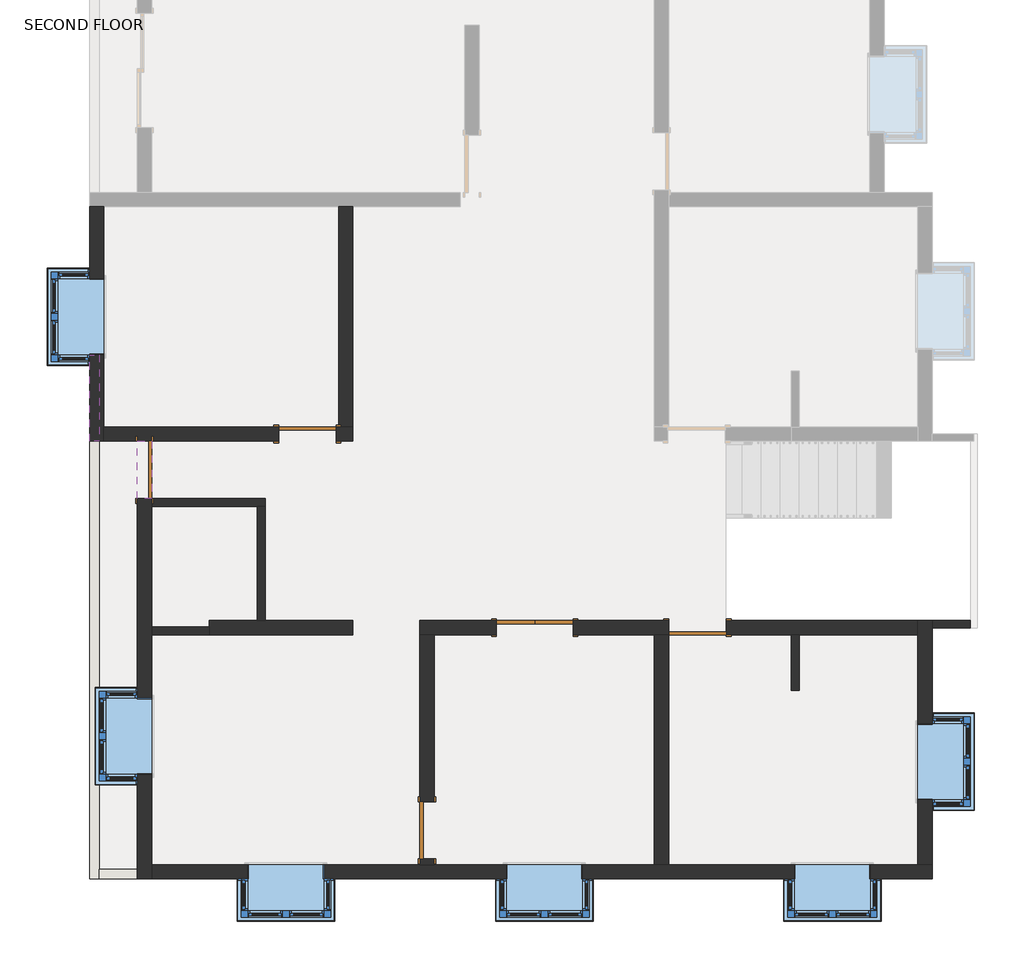
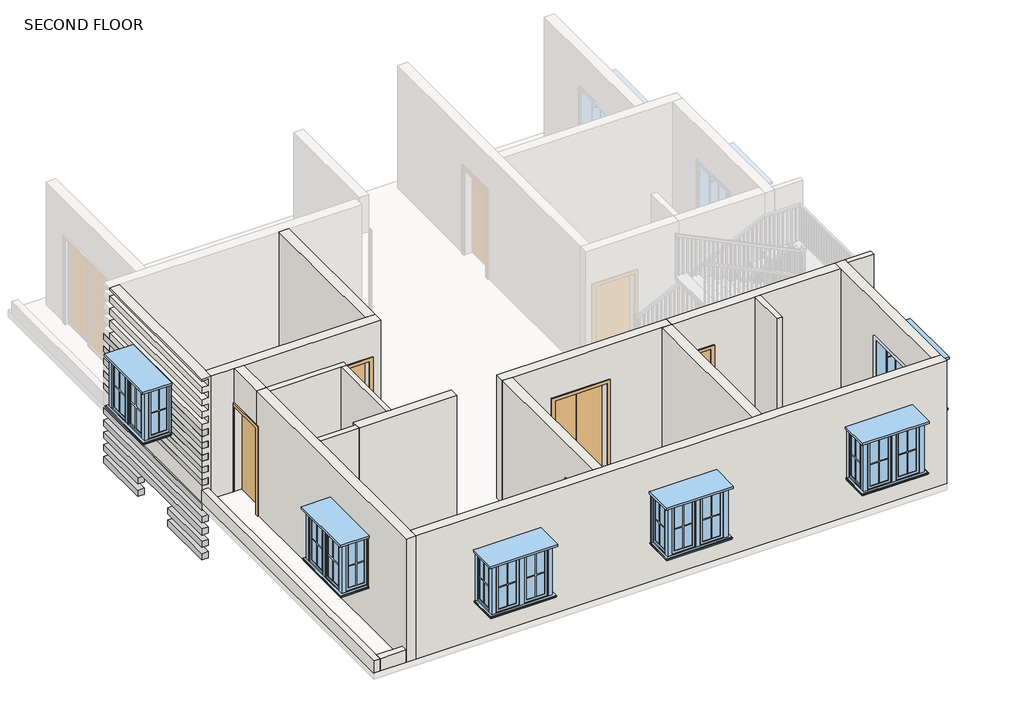
# One storey, part 1 of 6: 19 walls, 10 proxies, 6 windows, 5 doors.
"""IFC4 building model written with IfcOpenShell, lengths in millimetres."""

from ifc_helpers import new_model, si_unit, frame, origin, place, context, project, spatial, polyline, outline, extrude, faceted_brep, transform, mapped, element, save
from components import door_double_flush_panel_4_x7_7c704b5a, door_a90ba1ad, door_0ca8825f, window_bay_casement_box_90_degree_angle_4_x4_x2_07b705a1

model = new_model("IFC4")

# Units and contexts
model_context = context("Model", 3, world=origin())
ifc_project = project(units=[si_unit("LENGTHUNIT", "METRE", prefix="MILLI")], contexts=[model_context])

# Site, building, storey
site = spatial("IfcSite", under=ifc_project)
building = spatial("IfcBuilding", under=site)
storey = spatial("IfcBuildingStorey", under=building, Name="SECOND FLOOR", Elevation=6400.8)

# Proxies
placement = place(None, origin())
element("IfcBuildingElementProxy", 1, Name="Reveal", ObjectType="Reveal", at=placement, inside=storey, context=model_context, shape_type="SweptSolid", body=[
    extrude(outline(polyline([(-7008.3415084, 1592.333346), (-6855.9415084, 1592.333346), (-6855.9415084, 220.733346), (-7008.3415084, 220.733346), (-7008.3415084, 1592.333346)])), frame((0.0, 0.0, 4978.4), z_axis=(0.0, 0.0, 1.0), x_axis=(1.0, 0.0, 0.0)), (0.0, 0.0, 1.0), 152.4),
    extrude(outline(polyline([(-7008.3415084, 4183.133346), (-6855.9415084, 4183.133346), (-6855.9415084, 2811.533346), (-7008.3415084, 2811.533346), (-7008.3415084, 4183.133346)])), frame((0.0, 0.0, 4978.4), z_axis=(0.0, 0.0, 1.0), x_axis=(1.0, 0.0, 0.0)), (0.0, 0.0, 1.0), 152.4),
])
element("IfcBuildingElementProxy", 2, Name="Reveal", ObjectType="Reveal", at=placement, inside=storey, context=model_context, shape_type="SweptSolid", body=[
    extrude(outline(polyline([(-7008.3415084, 1592.333346), (-6855.9415084, 1592.333346), (-6855.9415084, 220.733346), (-7008.3415084, 220.733346), (-7008.3415084, 1592.333346)])), frame((0.0, 0.0, 5283.2), z_axis=(0.0, 0.0, 1.0), x_axis=(1.0, 0.0, 0.0)), (0.0, 0.0, 1.0), 152.4),
    extrude(outline(polyline([(-7008.3415084, 4183.133346), (-6855.9415084, 4183.133346), (-6855.9415084, 2811.533346), (-7008.3415084, 2811.533346), (-7008.3415084, 4183.133346)])), frame((0.0, 0.0, 5283.2), z_axis=(0.0, 0.0, 1.0), x_axis=(1.0, 0.0, 0.0)), (0.0, 0.0, 1.0), 152.4),
])
element("IfcBuildingElementProxy", 3, Name="Reveal", ObjectType="Reveal", at=placement, inside=storey, context=model_context, shape_type="SweptSolid", body=[
    extrude(outline(polyline([(-7008.3415084, 4183.133346), (-6855.9415084, 4183.133346), (-6855.9415084, 220.733346), (-7008.3415084, 220.733346), (-7008.3415084, 4183.133346)])), frame((0.0, 0.0, 5588.0), z_axis=(0.0, 0.0, 1.0), x_axis=(1.0, 0.0, 0.0)), (0.0, 0.0, 1.0), 152.4),
])
element("IfcBuildingElementProxy", 4, Name="Reveal", ObjectType="Reveal", at=placement, inside=storey, context=model_context, shape_type="SweptSolid", body=[
    extrude(outline(polyline([(-7008.3415084, 4183.133346), (-6855.9415084, 4183.133346), (-6855.9415084, 220.733346), (-7008.3415084, 220.733346), (-7008.3415084, 4183.133346)])), frame((0.0, 0.0, 5892.8), z_axis=(0.0, 0.0, 1.0), x_axis=(1.0, 0.0, 0.0)), (0.0, 0.0, 1.0), 152.4),
])
element("IfcBuildingElementProxy", 5, Name="Reveal", ObjectType="Reveal", at=placement, inside=storey, context=model_context, shape_type="SweptSolid", body=[
    extrude(outline(polyline([(-7008.3415084, 4183.133346), (-6855.9415084, 4183.133346), (-6855.9415084, 220.733346), (-7008.3415084, 220.733346), (-7008.3415084, 4183.133346)])), frame((0.0, 0.0, 6197.6), z_axis=(0.0, 0.0, 1.0), x_axis=(1.0, 0.0, 0.0)), (0.0, 0.0, 1.0), 152.4),
])
element("IfcBuildingElementProxy", 6, Name="Reveal", ObjectType="Reveal", at=placement, inside=storey, context=model_context, shape_type="SweptSolid", body=[
    extrude(outline(polyline([(-7008.3415084, 4183.133346), (-6855.9415084, 4183.133346), (-6855.9415084, 220.733346), (-7008.3415084, 220.733346), (-7008.3415084, 4183.133346)])), frame((0.0, 0.0, 6807.2), z_axis=(0.0, 0.0, 1.0), x_axis=(1.0, 0.0, 0.0)), (0.0, 0.0, 1.0), 152.4),
])
element("IfcBuildingElementProxy", 7, Name="Reveal", ObjectType="Reveal", at=placement, inside=storey, context=model_context, shape_type="SweptSolid", body=[
    extrude(outline(polyline([(-7008.3415084, 4183.133346), (-6855.9415084, 4183.133346), (-6855.9415084, 220.733346), (-7008.3415084, 220.733346), (-7008.3415084, 4183.133346)])), frame((0.0, 0.0, 7112.0), z_axis=(0.0, 0.0, 1.0), x_axis=(1.0, 0.0, 0.0)), (0.0, 0.0, 1.0), 152.4),
])
element("IfcBuildingElementProxy", 8, Name="Reveal", ObjectType="Reveal", at=placement, inside=storey, context=model_context, shape_type="SweptSolid", body=[
    extrude(outline(polyline([(-7008.3415084, 1592.333346), (-6855.9415084, 1592.333346), (-6855.9415084, 220.733346), (-7008.3415084, 220.733346), (-7008.3415084, 1592.333346)])), frame((0.0, 0.0, 7416.8), z_axis=(0.0, 0.0, 1.0), x_axis=(1.0, 0.0, 0.0)), (0.0, 0.0, 1.0), 152.4),
    extrude(outline(polyline([(-7008.3415084, 4183.133346), (-6855.9415084, 4183.133346), (-6855.9415084, 2811.533346), (-7008.3415084, 2811.533346), (-7008.3415084, 4183.133346)])), frame((0.0, 0.0, 7416.8), z_axis=(0.0, 0.0, 1.0), x_axis=(1.0, 0.0, 0.0)), (0.0, 0.0, 1.0), 152.4),
])
element("IfcBuildingElementProxy", 9, Name="Reveal", ObjectType="Reveal", at=placement, inside=storey, context=model_context, shape_type="SweptSolid", body=[
    extrude(outline(polyline([(-7008.3415084, 1592.333346), (-6855.9415084, 1592.333346), (-6855.9415084, 220.733346), (-7008.3415084, 220.733346), (-7008.3415084, 1592.333346)])), frame((0.0, 0.0, 7721.6), z_axis=(0.0, 0.0, 1.0), x_axis=(1.0, 0.0, 0.0)), (0.0, 0.0, 1.0), 152.4),
    extrude(outline(polyline([(-7008.3415084, 4183.133346), (-6855.9415084, 4183.133346), (-6855.9415084, 2811.533346), (-7008.3415084, 2811.533346), (-7008.3415084, 4183.133346)])), frame((0.0, 0.0, 7721.6), z_axis=(0.0, 0.0, 1.0), x_axis=(1.0, 0.0, 0.0)), (0.0, 0.0, 1.0), 152.4),
])
element("IfcBuildingElementProxy", 10, Name="Reveal", ObjectType="Reveal", at=placement, inside=storey, context=model_context, shape_type="SweptSolid", body=[
    extrude(outline(polyline([(-7008.3415084, 1592.333346), (-6855.9415084, 1592.333346), (-6855.9415084, 220.733346), (-7008.3415084, 220.733346), (-7008.3415084, 1592.333346)])), frame((0.0, 0.0, 8026.4), z_axis=(0.0, 0.0, 1.0), x_axis=(1.0, 0.0, 0.0)), (0.0, 0.0, 1.0), 152.4),
    extrude(outline(polyline([(-7008.3415084, 4183.133346), (-6855.9415084, 4183.133346), (-6855.9415084, 2811.533346), (-7008.3415084, 2811.533346), (-7008.3415084, 4183.133346)])), frame((0.0, 0.0, 8026.4), z_axis=(0.0, 0.0, 1.0), x_axis=(1.0, 0.0, 0.0)), (0.0, 0.0, 1.0), 152.4),
])

# Doors
door_double_flush_panel_4_x7_shape = door_double_flush_panel_4_x7_7c704b5a(model_context)
element("IfcDoor", 11, ObjectType="Door-Double-Flush_Panel : 4'x7'", at=placement, inside=storey, context=model_context, shape_type="MappedRepresentation", body=[
    mapped(door_double_flush_panel_4_x7_shape, transform((78.2584916, -2751.066654, 6400.8), x_axis=(1.0, 0.0, 0.0), y_axis=(0.0, 1.0, 0.0), z_axis=(0.0, 0.0, 1.0))),
])
door_shape = door_a90ba1ad(model_context)
element("IfcDoor", 12, ObjectType="Single-Flush : 36\" x 84\"", at=placement, inside=storey, context=model_context, shape_type="MappedRepresentation", body=[
    mapped(door_shape, transform((-1636.2415084, -5976.866654, 6400.8), x_axis=(0.0, -1.0, 0.0), y_axis=(1.0, 0.0, 0.0), z_axis=(0.0, 0.0, 1.0))),
])
door_2_shape = door_0ca8825f(model_context)
element("IfcDoor", 13, ObjectType="Single-Flush : 36\" x 84\"", at=placement, inside=storey, context=model_context, shape_type="MappedRepresentation", body=[
    mapped(door_2_shape, transform((-3541.2415084, 335.033346, 6400.8), x_axis=(1.0, 0.0, 0.0), y_axis=(0.0, 1.0, 0.0), z_axis=(0.0, 0.0, 1.0))),
])
element("IfcDoor", 14, ObjectType="Single-Flush : 36\" x 84\"", at=placement, inside=storey, context=model_context, shape_type="MappedRepresentation", body=[
    mapped(door_2_shape, transform((2669.0584916, -2751.066654, 6400.8), x_axis=(-1.0, 0.0, 0.0), y_axis=(0.0, -1.0, 0.0), z_axis=(0.0, 0.0, 1.0))),
])
element("IfcDoor", 15, ObjectType="Single-Flush : 36\" x 84\"", at=placement, inside=storey, context=model_context, shape_type="MappedRepresentation", body=[
    mapped(door_2_shape, transform((-6132.0415084, -236.466654, 6400.8), x_axis=(0.0, -1.0, 0.0), y_axis=(1.0, 0.0, 0.0), z_axis=(0.0, 0.0, 1.0))),
])

# Walls
element("IfcWall", 16, ObjectType="4.6\"", at=placement, inside=storey, context=model_context, shape_type="SweptSolid", body=[
    extrude(outline(polyline([(7009.1350459, -2753.606654), (6402.8584916, -2753.606654), (6402.8584916, -2636.766654), (7009.1350459, -2636.766654), (7009.1350459, -2753.606654)])), frame((0.0, 0.0, 6400.8), z_axis=(0.0, 0.0, 1.0), x_axis=(1.0, 0.0, 0.0)), (0.0, 0.0, 1.0), 3048.0),
])
element("IfcWall", 17, ObjectType="5\"", at=placement, inside=storey, context=model_context, shape_type="SweptSolid", body=[
    extrude(outline(polyline([(4159.1868368, -3751.826654), (4159.1868368, -2865.366654), (4286.1868368, -2865.366654), (4286.1868368, -3751.826654), (4159.1868368, -3751.826654)])), frame((0.0, 0.0, 6400.8), z_axis=(0.0, 0.0, 1.0), x_axis=(1.0, 0.0, 0.0)), (0.0, 0.0, 1.0), 3048.0),
])
element("IfcWall", 18, ObjectType="5\"", at=placement, inside=storey, context=model_context, shape_type="Brep", body=[
    faceted_brep([(-6017.7415084, -820.666654, 6400.8), (-4341.3415084, -820.666654, 6400.8), (-4214.3415084, -820.666654, 6400.8), (-4214.3415084, -820.666654, 9448.8), (-4341.3415084, -820.666654, 9448.8), (-6017.7415084, -820.666654, 9448.8), (-6017.7415084, -693.666654, 6400.8), (-6017.7415084, -693.666654, 9448.8), (-4214.3415084, -693.666654, 9448.8), (-4214.3415084, -693.666654, 6400.8)], [[[0, 1, 2, 3, 4, 5]], [[6, 7, 8, 9]], [[2, 1, 0, 6, 9]], [[5, 4, 3, 8, 7]], [[0, 5, 7, 6]], [[3, 2, 9, 8]]]),
])
element("IfcWall", 19, ObjectType="5\"", at=placement, inside=storey, context=model_context, shape_type="SweptSolid", body=[
    extrude(outline(polyline([(-4341.3415084, -2636.766654), (-4341.3415084, -820.666654), (-4214.3415084, -820.666654), (-4214.3415084, -2636.766654), (-4341.3415084, -2636.766654)])), frame((0.0, 0.0, 6400.8), z_axis=(0.0, 0.0, 1.0), x_axis=(1.0, 0.0, 0.0)), (0.0, 0.0, 1.0), 3048.0),
])
element("IfcWall", 20, ObjectType="5\"", at=placement, inside=storey, context=model_context, shape_type="SweptSolid", body=[
    extrude(outline(polyline([(-6017.7415084, -2738.366654), (-5103.3415084, -2738.366654), (-5103.3415084, -2865.366654), (-6017.7415084, -2865.366654), (-6017.7415084, -2738.366654)])), frame((0.0, 0.0, 6400.8), z_axis=(0.0, 0.0, 1.0), x_axis=(1.0, 0.0, 0.0)), (0.0, 0.0, 1.0), 3048.0),
])
element("IfcWall", 21, ObjectType="6\"", at=placement, inside=storey, context=model_context, shape_type="Brep", body=[
    faceted_brep([(-7008.3415084, 220.733346, 6400.8), (-7008.3415084, -6751.566654, 6400.8), (-7008.3415084, -6751.566654, 6705.6), (-7008.3415084, 220.733346, 6705.6), (-6855.9415084, 220.733346, 6400.8), (-6855.9415084, 220.733346, 6705.6), (-6855.9415084, -6599.166654, 6705.6), (-6855.9415084, -6751.566654, 6705.6), (-6855.9415084, -6751.566654, 6400.8), (-6855.9415084, -6599.166654, 6400.8)], [[[0, 1, 2, 3]], [[4, 5, 6, 7, 8, 9]], [[1, 0, 4, 9, 8]], [[3, 2, 7, 6, 5]], [[2, 1, 8, 7]], [[0, 3, 5, 4]]]),
])
element("IfcWall", 22, ObjectType="6\"", at=placement, inside=storey, context=model_context, shape_type="SweptSolid", body=[
    extrude(outline(polyline([(-6246.3415084, -6751.566654), (-6855.9415084, -6751.566654), (-6855.9415084, -6599.166654), (-6246.3415084, -6599.166654), (-6246.3415084, -6751.566654)])), frame((0.0, 0.0, 6400.8), z_axis=(0.0, 0.0, 1.0), x_axis=(1.0, 0.0, 0.0)), (0.0, 0.0, 1.0), 304.8),
])
element("IfcWall", 23, ObjectType="9\"", at=placement, inside=storey, context=model_context, shape_type="Brep", body=[
    faceted_brep([(-7008.3415084, 3954.533346, 6400.8), (-7008.3415084, 220.733346, 6400.8), (-7008.3415084, 220.733346, 6705.6), (-7008.3415084, 220.733346, 6807.2), (-7008.3415084, 3954.533346, 6807.2), (-7008.3415084, 220.733346, 9448.8), (-7008.3415084, 3954.533346, 9448.8), (-7008.3415084, 3954.533346, 9398.0), (-7008.3415084, 220.733346, 9398.0), (-7008.3415084, 1592.333346, 7315.2), (-7008.3415084, 2811.533346, 7315.2), (-7008.3415084, 2811.533346, 7416.8), (-7008.3415084, 3954.533346, 7416.8), (-7008.3415084, 3954.533346, 7264.4), (-7008.3415084, 220.733346, 7264.4), (-7008.3415084, 220.733346, 7416.8), (-7008.3415084, 1592.333346, 7416.8), (-7008.3415084, 2811.533346, 8585.2), (-7008.3415084, 1592.333346, 8585.2), (-7008.3415084, 1592.333346, 8483.6), (-7008.3415084, 220.733346, 8483.6), (-7008.3415084, 220.733346, 8636.0), (-7008.3415084, 3954.533346, 8636.0), (-7008.3415084, 3954.533346, 8483.6), (-7008.3415084, 2811.533346, 8483.6), (-7008.3415084, 220.733346, 9245.6), (-7008.3415084, 3954.533346, 9245.6), (-7008.3415084, 3954.533346, 9093.2), (-7008.3415084, 220.733346, 9093.2), (-7008.3415084, 220.733346, 8940.8), (-7008.3415084, 3954.533346, 8940.8), (-7008.3415084, 3954.533346, 8788.4), (-7008.3415084, 220.733346, 8788.4), (-7008.3415084, 220.733346, 8331.2), (-7008.3415084, 1592.333346, 8331.2), (-7008.3415084, 1592.333346, 8178.8), (-7008.3415084, 220.733346, 8178.8), (-7008.3415084, 2811.533346, 8331.2), (-7008.3415084, 3954.533346, 8331.2), (-7008.3415084, 3954.533346, 8178.8), (-7008.3415084, 2811.533346, 8178.8), (-7008.3415084, 220.733346, 8026.4), (-7008.3415084, 1592.333346, 8026.4), (-7008.3415084, 1592.333346, 7874.0), (-7008.3415084, 220.733346, 7874.0), (-7008.3415084, 2811.533346, 8026.4), (-7008.3415084, 3954.533346, 8026.4), (-7008.3415084, 3954.533346, 7874.0), (-7008.3415084, 2811.533346, 7874.0), (-7008.3415084, 220.733346, 7721.6), (-7008.3415084, 1592.333346, 7721.6), (-7008.3415084, 1592.333346, 7569.2), (-7008.3415084, 220.733346, 7569.2), (-7008.3415084, 2811.533346, 7721.6), (-7008.3415084, 3954.533346, 7721.6), (-7008.3415084, 3954.533346, 7569.2), (-7008.3415084, 2811.533346, 7569.2), (-7008.3415084, 220.733346, 7112.0), (-7008.3415084, 3954.533346, 7112.0), (-7008.3415084, 3954.533346, 6959.6), (-7008.3415084, 220.733346, 6959.6), (-6779.7415084, 220.733346, 6400.8), (-6779.7415084, 449.333346, 6400.8), (-6779.7415084, 3954.533346, 6400.8), (-6779.7415084, 3954.533346, 9448.8), (-6779.7415084, 449.333346, 9448.8), (-6779.7415084, 220.733346, 9448.8), (-6779.7415084, 2811.533346, 8585.2), (-6779.7415084, 2811.533346, 7315.2), (-6779.7415084, 1592.333346, 7315.2), (-6779.7415084, 1592.333346, 8585.2), (-6855.9415084, 220.733346, 6400.8), (-6855.9415084, 2811.533346, 8483.6), (-6855.9415084, 2811.533346, 8331.2), (-6855.9415084, 2811.533346, 8178.8), (-6855.9415084, 2811.533346, 8026.4), (-6855.9415084, 2811.533346, 7874.0), (-6855.9415084, 2811.533346, 7721.6), (-6855.9415084, 2811.533346, 7569.2), (-6855.9415084, 2811.533346, 7416.8), (-6855.9415084, 1592.333346, 7416.8), (-6855.9415084, 1592.333346, 7569.2), (-6855.9415084, 1592.333346, 7721.6), (-6855.9415084, 1592.333346, 7874.0), (-6855.9415084, 1592.333346, 8026.4), (-6855.9415084, 1592.333346, 8178.8), (-6855.9415084, 1592.333346, 8331.2), (-6855.9415084, 1592.333346, 8483.6), (-6855.9415084, 220.733346, 9398.0), (-6855.9415084, 220.733346, 9245.6), (-6855.9415084, 220.733346, 9093.2), (-6855.9415084, 220.733346, 8940.8), (-6855.9415084, 220.733346, 8788.4), (-6855.9415084, 220.733346, 8636.0), (-6855.9415084, 220.733346, 8483.6), (-6855.9415084, 220.733346, 8331.2), (-6855.9415084, 220.733346, 8178.8), (-6855.9415084, 220.733346, 8026.4), (-6855.9415084, 220.733346, 7874.0), (-6855.9415084, 220.733346, 7721.6), (-6855.9415084, 220.733346, 7569.2), (-6855.9415084, 220.733346, 7416.8), (-6855.9415084, 220.733346, 7264.4), (-6855.9415084, 220.733346, 7112.0), (-6855.9415084, 220.733346, 6959.6), (-6855.9415084, 220.733346, 6807.2), (-6855.9415084, 3954.533346, 6807.2), (-6855.9415084, 3954.533346, 6959.6), (-6855.9415084, 3954.533346, 7112.0), (-6855.9415084, 3954.533346, 7264.4), (-6855.9415084, 3954.533346, 7416.8), (-6855.9415084, 3954.533346, 7569.2), (-6855.9415084, 3954.533346, 7721.6), (-6855.9415084, 3954.533346, 7874.0), (-6855.9415084, 3954.533346, 8026.4), (-6855.9415084, 3954.533346, 8178.8), (-6855.9415084, 3954.533346, 8331.2), (-6855.9415084, 3954.533346, 8483.6), (-6855.9415084, 3954.533346, 8636.0), (-6855.9415084, 3954.533346, 8788.4), (-6855.9415084, 3954.533346, 8940.8), (-6855.9415084, 3954.533346, 9093.2), (-6855.9415084, 3954.533346, 9245.6), (-6855.9415084, 3954.533346, 9398.0)], [[[0, 1, 2, 3, 4]], [[5, 6, 7, 8]], [[9, 10, 11, 12, 13, 14, 15, 16]], [[17, 18, 19, 20, 21, 22, 23, 24]], [[25, 26, 27, 28]], [[29, 30, 31, 32]], [[33, 34, 35, 36]], [[37, 38, 39, 40]], [[41, 42, 43, 44]], [[45, 46, 47, 48]], [[49, 50, 51, 52]], [[53, 54, 55, 56]], [[57, 58, 59, 60]], [[61, 62, 63, 64, 65, 66], [67, 68, 69, 70]], [[1, 0, 63, 62, 61, 71]], [[6, 5, 66, 65, 64]], [[68, 67, 17, 24, 72, 73, 37, 40, 74, 75, 45, 48, 76, 77, 53, 56, 78, 79, 11, 10]], [[69, 68, 10, 9]], [[70, 69, 9, 16, 80, 81, 51, 50, 82, 83, 43, 42, 84, 85, 35, 34, 86, 87, 19, 18]], [[67, 70, 18, 17]], [[1, 71, 61, 66, 5, 8, 88, 89, 25, 28, 90, 91, 29, 32, 92, 93, 21, 20, 94, 95, 33, 36, 96, 97, 41, 44, 98, 99, 49, 52, 100, 101, 15, 14, 102, 103, 57, 60, 104, 105, 3, 2]], [[6, 64, 63, 0, 4, 106, 107, 59, 58, 108, 109, 13, 12, 110, 111, 55, 54, 112, 113, 47, 46, 114, 115, 39, 38, 116, 117, 23, 22, 118, 119, 31, 30, 120, 121, 27, 26, 122, 123, 7]], [[123, 88, 8, 7]], [[88, 123, 122, 89]], [[89, 122, 26, 25]], [[121, 90, 28, 27]], [[90, 121, 120, 91]], [[91, 120, 30, 29]], [[119, 92, 32, 31]], [[92, 119, 118, 93]], [[93, 118, 22, 21]], [[87, 94, 20, 19]], [[94, 87, 86, 95]], [[95, 86, 34, 33]], [[117, 72, 24, 23]], [[72, 117, 116, 73]], [[73, 116, 38, 37]], [[85, 96, 36, 35]], [[96, 85, 84, 97]], [[97, 84, 42, 41]], [[115, 74, 40, 39]], [[74, 115, 114, 75]], [[75, 114, 46, 45]], [[83, 98, 44, 43]], [[98, 83, 82, 99]], [[99, 82, 50, 49]], [[113, 76, 48, 47]], [[76, 113, 112, 77]], [[77, 112, 54, 53]], [[81, 100, 52, 51]], [[100, 81, 80, 101]], [[101, 80, 16, 15]], [[111, 78, 56, 55]], [[78, 111, 110, 79]], [[79, 110, 12, 11]], [[109, 102, 14, 13]], [[102, 109, 108, 103]], [[103, 108, 58, 57]], [[107, 104, 60, 59]], [[104, 107, 106, 105]], [[105, 106, 4, 3]]]),
])
element("IfcWall", 24, ObjectType="9\"", at=placement, inside=storey, context=model_context, shape_type="Brep", body=[
    faceted_brep([(-3084.0415084, 220.733346, 8534.4), (-3084.0415084, 220.733346, 6400.8), (-2817.3415084, 220.733346, 6400.8), (-2817.3415084, 220.733346, 9448.8), (-6017.7415084, 220.733346, 9448.8), (-6246.3415084, 220.733346, 9448.8), (-6779.7415084, 220.733346, 9448.8), (-6779.7415084, 220.733346, 6400.8), (-3998.4415084, 220.733346, 6400.8), (-3998.4415084, 220.733346, 8534.4), (-2817.3415084, 449.333346, 6400.8), (-3045.9415084, 449.333346, 6400.8), (-3084.0415084, 449.333346, 6400.8), (-3084.0415084, 449.333346, 8534.4), (-3998.4415084, 449.333346, 8534.4), (-3998.4415084, 449.333346, 6400.8), (-6779.7415084, 449.333346, 6400.8), (-6779.7415084, 449.333346, 9448.8), (-3045.9415084, 449.333346, 9448.8), (-2817.3415084, 449.333346, 9448.8)], [[[0, 1, 2, 3, 4, 5, 6, 7, 8, 9]], [[10, 11, 12, 13, 14, 15, 16, 17, 18, 19]], [[8, 7, 16, 15]], [[2, 1, 12, 11, 10]], [[6, 5, 4, 3, 19, 18, 17]], [[3, 2, 10, 19]], [[13, 12, 1, 0]], [[14, 13, 0, 9]], [[15, 14, 9, 8]], [[6, 17, 16, 7]]]),
])
element("IfcWall", 25, ObjectType="9\"", at=placement, inside=storey, context=model_context, shape_type="SweptSolid", body=[
    extrude(outline(polyline([(-2817.3415084, 3954.533346), (-2817.3415084, 449.333346), (-3045.9415084, 449.333346), (-3045.9415084, 3954.533346), (-2817.3415084, 3954.533346)])), frame((0.0, 0.0, 6400.8), z_axis=(0.0, 0.0, 1.0), x_axis=(1.0, 0.0, 0.0)), (0.0, 0.0, 1.0), 3048.0),
])
element("IfcWall", 26, ObjectType="9\"", at=placement, inside=storey, context=model_context, shape_type="Brep", body=[
    faceted_brep([(-6246.3415084, -693.666654, 6400.8), (-6246.3415084, -6599.166654, 6400.8), (-6246.3415084, -6751.566654, 6400.8), (-6246.3415084, -6751.566654, 6705.6), (-6246.3415084, -6751.566654, 9448.8), (-6246.3415084, -693.666654, 9448.8), (-6246.3415084, -693.666654, 8534.4), (-6246.3415084, -3868.666654, 8585.2), (-6246.3415084, -5087.866654, 8585.2), (-6246.3415084, -5087.866654, 7315.2), (-6246.3415084, -3868.666654, 7315.2), (-6017.7415084, -693.666654, 6400.8), (-6017.7415084, -693.666654, 8534.4), (-6017.7415084, -693.666654, 9448.8), (-6017.7415084, -820.666654, 9448.8), (-6017.7415084, -2738.366654, 9448.8), (-6017.7415084, -2865.366654, 9448.8), (-6017.7415084, -6522.966654, 9448.8), (-6017.7415084, -6751.566654, 9448.8), (-6017.7415084, -6751.566654, 6400.8), (-6017.7415084, -6522.966654, 6400.8), (-6017.7415084, -2865.366654, 6400.8), (-6017.7415084, -2738.366654, 6400.8), (-6017.7415084, -820.666654, 6400.8), (-6017.7415084, -3868.666654, 8585.2), (-6017.7415084, -3868.666654, 7315.2), (-6017.7415084, -5087.866654, 7315.2), (-6017.7415084, -5087.866654, 8585.2)], [[[0, 1, 2, 3, 4, 5, 6], [7, 8, 9, 10]], [[11, 12, 13, 14, 15, 16, 17, 18, 19, 20, 21, 22, 23], [24, 25, 26, 27]], [[2, 1, 0, 11, 23, 22, 21, 20, 19]], [[5, 4, 18, 17, 16, 15, 14, 13]], [[0, 6, 5, 13, 12, 11]], [[25, 24, 7, 10]], [[26, 25, 10, 9]], [[27, 26, 9, 8]], [[24, 27, 8, 7]], [[2, 19, 18, 4, 3]]]),
])
element("IfcWall", 27, ObjectType="9\"", at=placement, inside=storey, context=model_context, shape_type="Brep", body=[
    faceted_brep([(-2817.3415084, -2636.766654, 6400.8), (-4214.3415084, -2636.766654, 6400.8), (-4341.3415084, -2636.766654, 6400.8), (-5103.3415084, -2636.766654, 6400.8), (-5103.3415084, -2636.766654, 9448.8), (-4341.3415084, -2636.766654, 9448.8), (-4214.3415084, -2636.766654, 9448.8), (-2817.3415084, -2636.766654, 9448.8), (-2817.3415084, -2865.366654, 6400.8), (-2817.3415084, -2865.366654, 9448.8), (-5103.3415084, -2865.366654, 9448.8), (-5103.3415084, -2865.366654, 6400.8), (-5103.3415084, -2738.366654, 6400.8), (-5103.3415084, -2738.366654, 9448.8)], [[[0, 1, 2, 3, 4, 5, 6, 7]], [[8, 9, 10, 11]], [[3, 2, 1, 0, 8, 11, 12]], [[4, 3, 12, 11, 10, 13]], [[7, 6, 5, 4, 13, 10, 9]], [[0, 7, 9, 8]]]),
])
element("IfcWall", 28, ObjectType="9\"", at=placement, inside=storey, context=model_context, shape_type="Brep", body=[
    faceted_brep([(2211.8584916, -2865.366654, 9448.8), (1983.2584916, -2865.366654, 9448.8), (-1521.9415084, -2865.366654, 9448.8), (-1750.5415084, -2865.366654, 9448.8), (-1750.5415084, -2865.366654, 6400.8), (-1521.9415084, -2865.366654, 6400.8), (-531.3415084, -2865.366654, 6400.8), (-531.3415084, -2865.366654, 8534.4), (687.8584916, -2865.366654, 8534.4), (687.8584916, -2865.366654, 6400.8), (1983.2584916, -2865.366654, 6400.8), (2211.8584916, -2865.366654, 6400.8), (2211.8584916, -2865.366654, 8534.4), (-1750.5415084, -2636.766654, 9448.8), (2211.8584916, -2636.766654, 9448.8), (2211.8584916, -2636.766654, 8534.4), (2211.8584916, -2636.766654, 6400.8), (687.8584916, -2636.766654, 6400.8), (687.8584916, -2636.766654, 8534.4), (-531.3415084, -2636.766654, 8534.4), (-531.3415084, -2636.766654, 6400.8), (-1750.5415084, -2636.766654, 6400.8)], [[[0, 1, 2, 3, 4, 5, 6, 7, 8, 9, 10, 11, 12]], [[13, 14, 15, 16, 17, 18, 19, 20, 21]], [[16, 11, 10, 9, 17]], [[4, 21, 20, 6, 5]], [[3, 2, 1, 0, 14, 13]], [[0, 12, 11, 16, 15, 14]], [[4, 3, 13, 21]], [[8, 18, 17, 9]], [[18, 8, 7, 19]], [[19, 7, 6, 20]]]),
])
element("IfcWall", 29, ObjectType="9\"", at=placement, inside=storey, context=model_context, shape_type="SweptSolid", body=[
    extrude(outline(polyline([(1983.2584916, -6522.966654), (1983.2584916, -2865.366654), (2211.8584916, -2865.366654), (2211.8584916, -6522.966654), (1983.2584916, -6522.966654)])), frame((0.0, 0.0, 6400.8), z_axis=(0.0, 0.0, 1.0), x_axis=(1.0, 0.0, 0.0)), (0.0, 0.0, 1.0), 3048.0),
])
element("IfcWall", 30, ObjectType="9\"", at=placement, inside=storey, context=model_context, shape_type="Brep", body=[
    faceted_brep([(-6017.7415084, -6751.566654, 9448.8), (-6017.7415084, -6751.566654, 6400.8), (6402.8584916, -6751.566654, 6400.8), (6402.8584916, -6751.566654, 9448.8), (-378.9415084, -6751.566654, 8585.2), (840.2584916, -6751.566654, 8585.2), (840.2584916, -6751.566654, 7315.2), (-378.9415084, -6751.566654, 7315.2), (4205.7584916, -6751.566654, 8585.2), (5424.9584916, -6751.566654, 8585.2), (5424.9584916, -6751.566654, 7315.2), (4205.7584916, -6751.566654, 7315.2), (-4493.7415084, -6751.566654, 8585.2), (-3274.5415084, -6751.566654, 8585.2), (-3274.5415084, -6751.566654, 7315.2), (-4493.7415084, -6751.566654, 7315.2), (-6017.7415084, -6522.966654, 6400.8), (-6017.7415084, -6522.966654, 9448.8), (-1750.5415084, -6522.966654, 9448.8), (-1521.9415084, -6522.966654, 9448.8), (1983.2584916, -6522.966654, 9448.8), (2211.8584916, -6522.966654, 9448.8), (6174.2584916, -6522.966654, 9448.8), (6402.8584916, -6522.966654, 9448.8), (6402.8584916, -6522.966654, 6400.8), (6174.2584916, -6522.966654, 6400.8), (2211.8584916, -6522.966654, 6400.8), (1983.2584916, -6522.966654, 6400.8), (-1521.9415084, -6522.966654, 6400.8), (-1750.5415084, -6522.966654, 6400.8), (-378.9415084, -6522.966654, 8585.2), (-378.9415084, -6522.966654, 7315.2), (840.2584916, -6522.966654, 7315.2), (840.2584916, -6522.966654, 8585.2), (4205.7584916, -6522.966654, 8585.2), (4205.7584916, -6522.966654, 7315.2), (5424.9584916, -6522.966654, 7315.2), (5424.9584916, -6522.966654, 8585.2), (-4493.7415084, -6522.966654, 8585.2), (-4493.7415084, -6522.966654, 7315.2), (-3274.5415084, -6522.966654, 7315.2), (-3274.5415084, -6522.966654, 8585.2)], [[[0, 1, 2, 3], [4, 5, 6, 7], [8, 9, 10, 11], [12, 13, 14, 15]], [[16, 17, 18, 19, 20, 21, 22, 23, 24, 25, 26, 27, 28, 29], [30, 31, 32, 33], [34, 35, 36, 37], [38, 39, 40, 41]], [[2, 1, 16, 29, 28, 27, 26, 25, 24]], [[0, 3, 23, 22, 21, 20, 19, 18, 17]], [[3, 2, 24, 23]], [[31, 30, 4, 7]], [[32, 31, 7, 6]], [[33, 32, 6, 5]], [[30, 33, 5, 4]], [[35, 34, 8, 11]], [[36, 35, 11, 10]], [[37, 36, 10, 9]], [[34, 37, 9, 8]], [[39, 38, 12, 15]], [[40, 39, 15, 14]], [[41, 40, 14, 13]], [[38, 41, 13, 12]], [[0, 17, 16, 1]]]),
])
element("IfcWall", 31, ObjectType="9\"", at=placement, inside=storey, context=model_context, shape_type="Brep", body=[
    faceted_brep([(6402.8584916, -6522.966654, 6400.8), (6402.8584916, -2753.606654, 6400.8), (6402.8584916, -2636.766654, 6400.8), (6402.8584916, -2636.766654, 9448.8), (6402.8584916, -2753.606654, 9448.8), (6402.8584916, -6522.966654, 9448.8), (6402.8584916, -5494.266654, 8585.2), (6402.8584916, -4275.066654, 8585.2), (6402.8584916, -4275.066654, 7315.2), (6402.8584916, -5494.266654, 7315.2), (6174.2584916, -6522.966654, 6400.8), (6174.2584916, -6522.966654, 9448.8), (6174.2584916, -2865.366654, 9448.8), (6174.2584916, -2636.766654, 9448.8), (6174.2584916, -2636.766654, 6400.8), (6174.2584916, -2865.366654, 6400.8), (6174.2584916, -5494.266654, 8585.2), (6174.2584916, -5494.266654, 7315.2), (6174.2584916, -4275.066654, 7315.2), (6174.2584916, -4275.066654, 8585.2)], [[[0, 1, 2, 3, 4, 5], [6, 7, 8, 9]], [[10, 11, 12, 13, 14, 15], [16, 17, 18, 19]], [[2, 1, 0, 10, 15, 14]], [[5, 4, 3, 13, 12, 11]], [[0, 5, 11, 10]], [[3, 2, 14, 13]], [[17, 16, 6, 9]], [[18, 17, 9, 8]], [[19, 18, 8, 7]], [[16, 19, 7, 6]]]),
])
element("IfcWall", 32, ObjectType="9\"", at=placement, inside=storey, context=model_context, shape_type="Brep", body=[
    faceted_brep([(2211.8584916, -2636.766654, 9448.8), (6174.2584916, -2636.766654, 9448.8), (6174.2584916, -2636.766654, 6400.8), (3126.2584916, -2636.766654, 6400.8), (3126.2584916, -2636.766654, 8534.4), (2211.8584916, -2636.766654, 8534.4), (6174.2584916, -2865.366654, 9448.8), (4286.1868368, -2865.366654, 9448.8), (4159.1868368, -2865.366654, 9448.8), (2211.8584916, -2865.366654, 9448.8), (2211.8584916, -2865.366654, 8534.4), (3126.2584916, -2865.366654, 8534.4), (3126.2584916, -2865.366654, 6400.8), (4159.1868368, -2865.366654, 6400.8), (4286.1868368, -2865.366654, 6400.8), (6174.2584916, -2865.366654, 6400.8)], [[[0, 1, 2, 3, 4, 5]], [[6, 7, 8, 9, 10, 11, 12, 13, 14, 15]], [[2, 15, 14, 13, 12, 3]], [[1, 0, 9, 8, 7, 6]], [[2, 1, 6, 15]], [[9, 0, 5, 10]], [[4, 11, 10, 5]], [[11, 4, 3, 12]]]),
])
element("IfcWall", 33, ObjectType="9\"", at=placement, inside=storey, context=model_context, shape_type="SweptSolid", body=[
    extrude(outline(polyline([(-6434.066654, 8534.4), (-6434.066654, 6400.8), (-6522.966654, 6400.8), (-6522.966654, 9448.8), (-2865.366654, 9448.8), (-2865.366654, 6400.8), (-5519.666654, 6400.8), (-5519.666654, 8534.4), (-6434.066654, 8534.4)])), frame((-1750.5415084, 0.0, 0.0), z_axis=(1.0, 0.0, 0.0), x_axis=(0.0, 1.0, 0.0)), (0.0, 0.0, 1.0), 228.6),
])
element("IfcWall", 34, ObjectType="9\"", at=placement, inside=storey, context=model_context, shape_type="SweptSolid", body=[
    extrude(outline(polyline([(-6017.7415084, 220.733346), (-6017.7415084, -693.666654), (-6246.3415084, -693.666654), (-6246.3415084, 220.733346), (-6017.7415084, 220.733346)])), frame((0.0, 0.0, 8534.4), z_axis=(0.0, 0.0, 1.0), x_axis=(1.0, 0.0, 0.0)), (0.0, 0.0, 1.0), 914.4),
])

# Windows
window_bay_casement_box_90_degree_angle_4_x4_x2_shape = window_bay_casement_box_90_degree_angle_4_x4_x2_07b705a1(model_context)
element("IfcWindow", 35, ObjectType="Window-Bay-Casement-Box-90_Degree_Angle : 4'X4'X2'", at=placement, inside=storey, context=model_context, shape_type="MappedRepresentation", body=[
    mapped(window_bay_casement_box_90_degree_angle_4_x4_x2_shape, transform((-6894.0415084, 2201.933346, 6705.6), x_axis=(0.0, 1.0, 0.0), y_axis=(-1.0, 0.0, 0.0), z_axis=(0.0, 0.0, 1.0))),
])
element("IfcWindow", 36, ObjectType="Window-Bay-Casement-Box-90_Degree_Angle : 4'X4'X2'", at=placement, inside=storey, context=model_context, shape_type="MappedRepresentation", body=[
    mapped(window_bay_casement_box_90_degree_angle_4_x4_x2_shape, transform((-6132.0415084, -4478.266654, 6705.6), x_axis=(0.0, 1.0, 0.0), y_axis=(-1.0, 0.0, 0.0), z_axis=(0.0, 0.0, 1.0))),
])
element("IfcWindow", 37, ObjectType="Window-Bay-Casement-Box-90_Degree_Angle : 4'X4'X2'", at=placement, inside=storey, context=model_context, shape_type="MappedRepresentation", body=[
    mapped(window_bay_casement_box_90_degree_angle_4_x4_x2_shape, transform((6288.5584916, -4884.666654, 6705.6), x_axis=(0.0, -1.0, 0.0), y_axis=(1.0, 0.0, 0.0), z_axis=(0.0, 0.0, 1.0))),
])
element("IfcWindow", 38, ObjectType="Window-Bay-Casement-Box-90_Degree_Angle : 4'X4'X2'", at=placement, inside=storey, context=model_context, shape_type="MappedRepresentation", body=[
    mapped(window_bay_casement_box_90_degree_angle_4_x4_x2_shape, transform((230.6584916, -6637.266654, 6705.6), x_axis=(-1.0, 0.0, 0.0), y_axis=(0.0, -1.0, 0.0), z_axis=(0.0, 0.0, 1.0))),
])
element("IfcWindow", 39, ObjectType="Window-Bay-Casement-Box-90_Degree_Angle : 4'X4'X2'", at=placement, inside=storey, context=model_context, shape_type="MappedRepresentation", body=[
    mapped(window_bay_casement_box_90_degree_angle_4_x4_x2_shape, transform((4815.3584916, -6637.266654, 6705.6), x_axis=(-1.0, 0.0, 0.0), y_axis=(0.0, -1.0, 0.0), z_axis=(0.0, 0.0, 1.0))),
])
element("IfcWindow", 40, ObjectType="Window-Bay-Casement-Box-90_Degree_Angle : 4'X4'X2'", at=placement, inside=storey, context=model_context, shape_type="MappedRepresentation", body=[
    mapped(window_bay_casement_box_90_degree_angle_4_x4_x2_shape, transform((-3884.1415084, -6637.266654, 6705.6), x_axis=(-1.0, 0.0, 0.0), y_axis=(0.0, -1.0, 0.0), z_axis=(0.0, 0.0, 1.0))),
])

save(model, "model.ifc")

# Revit data of these elements
# Type "Door-Double-Flush_Panel : 4'x7'"
#   Type Mark = "9"
#   Construction Type Id = "DOOR"
#   Assembly Code = "C1020"
#   Analytic Construction = "Wooden"
#   Thickness = 0' - 2"
#   Thermal Resistance (R) = 2.5876 (h·ft²·°F)/BTU
#   Swing Angle [instance default] = 90.00°
#   Panel Width = 2' - 0"
#   Heat Transfer Coefficient (U) = 0.3865 BTU/(h·ft²·°F)
#   Height = 7' - 0"
#   Trim Projection Ext = 0' - 1"
#   Trim Projection Int = 0' - 1"
#   Trim Width = 0' - 3"
#   Width = 4' - 0"
#   Define Thermal Properties by = 1
#   Panel Material = Wood - Birch - Solid Stained Light Low Gloss
#   Trim Material = Paint - Sienna
#   Visual Light Transmittance = 0
#   Solar Heat Gain Coefficient = 0
#   Function = (empty or 0)
#   Wall Closure = (empty or 0)
# Type "Single-Flush : 36\" x 84\""
#   Type Mark = "1"
#   Construction Type Id = "MDOOR"
#   Assembly Code = "C1020"
#   Analytic Construction = "Metal"
#   Thickness = 0' - 2"
#   Heat Transfer Coefficient (U) = 0.651978 BTU/(h·ft²·°F)
#   Height = 7' - 0"
#   Trim Projection Ext = 0' - 1"
#   Trim Projection Int = 0' - 1"
#   Trim Width = 0' - 3"
#   Width = 3' - 0"
#   Define Thermal Properties by = 1
#   Define Thermal Properties by = 1
#   Door Material = Door - Panel
#   Frame Material = Door - Frame
#   Visual Light Transmittance = 0
#   Solar Heat Gain Coefficient = 0
#   Function = (empty or 0)
#   Wall Closure = (empty or 0)
# Type "4.6\""
#   Assembly Code = "B2010"
#   Layers, outside or top first: 0' - 4 77/128" no material (function 1)
# Type "5\""
#   Assembly Code = "B2010"
#   Layers, outside or top first: 0' - 5" no material (function 1)
# Type "6\""
#   Assembly Code = "B2010"
#   Layers, outside or top first: 0' - 6" no material (function 1)
# Type "9\""
#   Assembly Code = "B2010"
#   Layers, outside or top first: 0' - 9" "WALL 1" (function 1)
# Type "Window-Bay-Casement-Box-90_Degree_Angle : 4'X4'X2'"
#   Type Mark = "20"
#   Fire Rating = "0.5h"
#   Assembly Code = "B2020100"
#   Analytic Construction = "1/8 in Pilkington single glazing"
#   Width = 4' - 0"
#   Wall Thickness [instance default] = 0' - 6"
#   Visual Light Transmittance = 0.9
#   Trim Width = 4' - 8"
#   Trim Height = 4' - 0"
#   Thermal Resistance (R) = 1.5394 (h·ft²·°F)/BTU
#   Solar Heat Gain Coefficient = 0.86
#   Rough Width = 4' - 0 1/2"
#   Rough Height = 4' - 0 1/2"
#   Height 1 = 4' - 2"
#   Height = 4' - 0"
#   Heat Transfer Coefficient (U) = 0.6496 BTU/(h·ft²·°F)
#   Depth = 2' - 0"
#   Default Sill Height = 2' - 0"
#   Muntin Visibility = yes
#   Interior Trim Visibility [instance default] = yes
#   Exterior Trim Visibility [instance default] = yes
#   Muntin Pattern = Muntin Pattern_2x2 : Muntin Pattern_2x2
#   Interior Trim Material = Wood - Stained
#   Exterior Trim Material = Clad - White
#   Exterior Trim = element 423684
#   Interior Trim = Trim-Window-Interior-Flat : Picture Frame
#   Interior Frame Material = Wood - Stained
#   Glass Panel Material = Glass
#   Exterior Frame Material = Clad - White
#   Wall Closure = (empty or 0)
# Element 11 (IfcDoor, "Door-Double-Flush_Panel : 4'x7'")
#   Swing Angle = 90.00°
#   Phase Created = New Construction
#   Materials on its faces: "Paint - Sienna", "Wood - Birch - Solid Stained Light Low Gloss"
# Elements 12, 13, 14, 15 (IfcDoor, "Single-Flush : 36\" x 84\"")
#   Phase Created = New Construction
#   Materials on its faces: "Door - Frame", "Door - Panel"
# Element 16 (IfcWall, "4.6\"")
#   Top Offset = -0' - 6"
#   Base Offset = 0' - 0"
#   wall height = 10' - 0"
#   Phase Created = New Construction
#   Base Constraint = SECOND FLOOR
#   Top Constraint = THIRD FLOOR
#   Materials on its faces: "Default Wall", "WALL 2"
# Elements 17, 18, 19, 20 (IfcWall, "5\"")
#   Top Offset = -0' - 6"
#   Base Offset = 0' - 0"
#   wall height = 10' - 0"
#   Phase Created = New Construction
#   Base Constraint = SECOND FLOOR
#   Top Constraint = THIRD FLOOR
#   Materials on its faces: "Default Wall"
# Elements 21, 22 (IfcWall, "6\"")
#   Top Offset = -0' - 6"
#   Base Offset = 0' - 0"
#   Unconnected Height = 1' - 0"
#   wall height = 1' - 0"
#   Phase Created = New Construction
#   Base Constraint = SECOND FLOOR
#   Materials on its faces: "Default Wall", "WALL 4"
# Elements 23, 30, 31, 34 (IfcWall, "9\"")
#   Top Offset = -0' - 6"
#   Base Offset = 0' - 0"
#   wall height = 10' - 0"
#   Phase Created = New Construction
#   Base Constraint = SECOND FLOOR
#   Top Constraint = THIRD FLOOR
#   Materials on its faces: "WALL 1", "WALL 2"
# Elements 24, 25, 27, 28, 29, 32, 33 (IfcWall, "9\"")
#   Top Offset = -0' - 6"
#   Base Offset = 0' - 0"
#   wall height = 10' - 0"
#   Phase Created = New Construction
#   Base Constraint = SECOND FLOOR
#   Top Constraint = THIRD FLOOR
#   Materials on its faces: "WALL 1"
# Element 26 (IfcWall, "9\"")
#   Top Offset = -0' - 6"
#   Base Offset = 0' - 0"
#   wall height = 10' - 0"
#   Phase Created = New Construction
#   Base Constraint = SECOND FLOOR
#   Top Constraint = THIRD FLOOR
#   Materials on its faces: "WALL 1", "WALL 2", "Default Wall"
# Element 35 (IfcWindow, "Window-Bay-Casement-Box-90_Degree_Angle : 4'X4'X2'")
#   Mark = "29"
#   Phase Created = New Construction
#   Materials on its faces: "Clad - White", "Wood - Stained", "Glass"
# Element 36 (IfcWindow, "Window-Bay-Casement-Box-90_Degree_Angle : 4'X4'X2'")
#   Mark = "30"
#   Phase Created = New Construction
#   Materials on its faces: "Clad - White", "Wood - Stained", "Glass"
# Element 37 (IfcWindow, "Window-Bay-Casement-Box-90_Degree_Angle : 4'X4'X2'")
#   Mark = "31"
#   Phase Created = New Construction
#   Materials on its faces: "Clad - White", "Wood - Stained", "Glass"
# Element 38 (IfcWindow, "Window-Bay-Casement-Box-90_Degree_Angle : 4'X4'X2'")
#   Mark = "36"
#   Phase Created = New Construction
#   Materials on its faces: "Clad - White", "Wood - Stained", "Glass"
# Element 39 (IfcWindow, "Window-Bay-Casement-Box-90_Degree_Angle : 4'X4'X2'")
#   Mark = "37"
#   Phase Created = New Construction
#   Materials on its faces: "Clad - White", "Wood - Stained", "Glass"
# Element 40 (IfcWindow, "Window-Bay-Casement-Box-90_Degree_Angle : 4'X4'X2'")
#   Mark = "38"
#   Phase Created = New Construction
#   Materials on its faces: "Clad - White", "Wood - Stained", "Glass"
# Materials
#   "Wood - Birch - Solid Stained Light Low Gloss": class "Wood", colour RGB 210 159 95, transparency 0, Cost = 0
#   "Paint - Sienna": colour RGB 118 70 51, transparency 0, Cost = 0
#   "Door - Panel": class "Wood", colour RGB 210 159 95, transparency 0, Cost = 0
#   "Door - Frame": colour RGB 118 70 51, transparency 0, Cost = 0
#   "WALL 1": class "Generic", colour RGB 233 224 215, transparency 0, Cost = 0
#   "Wood - Stained": class "Wood", colour RGB 224 178 126, transparency 0, Cost = 0
#   "Clad - White": class "Wood", colour RGB 242 242 238, transparency 0, Cost = 0
#   "Glass": class "Glass", colour RGB 0 128 192, transparency 0.75, Description = "Soda Lime Glass", Cost = 0
#   "Default Wall": colour RGB 128 128 128, transparency 0, Cost = 0
#   "WALL 2": class "Generic", colour RGB 52 58 64, transparency 0, Cost = 0
#   "WALL 4": class "Generic", colour RGB 32 32 32, transparency 0, Cost = 0
